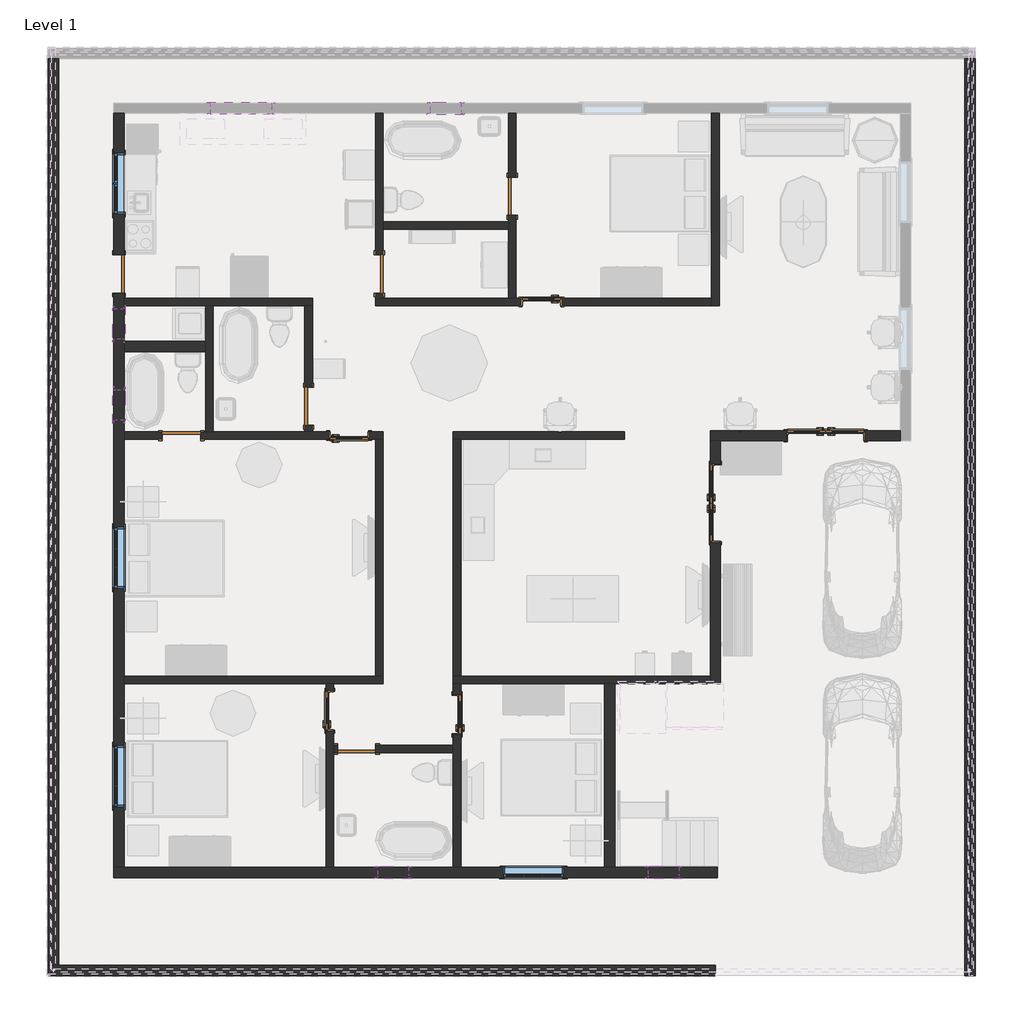
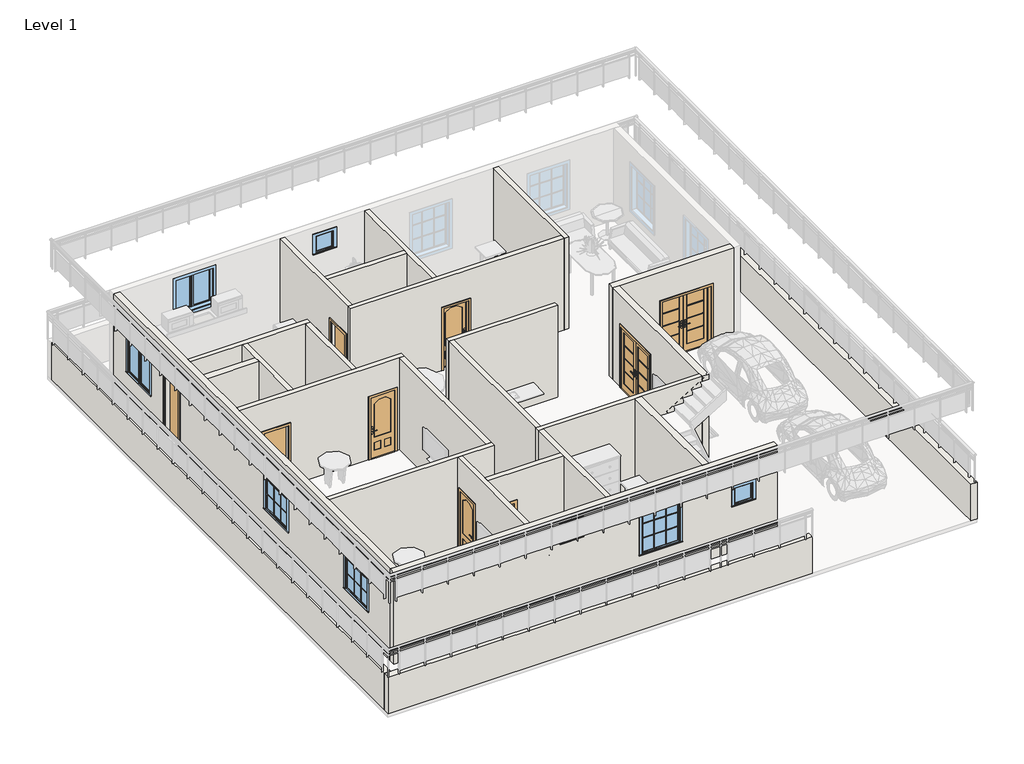
# One storey, part 1 of 6: 26 walls, 12 doors, 10 windows.
"""IFC4 building model written with IfcOpenShell, lengths in millimetres."""

from ifc_helpers import new_model, si_unit, frame, origin, origin_with_axes, place, context, project, spatial, polyline, outline, extrude, faceted_brep, transform, mapped, element, save
from components import door_14b9be53, door_4b146b56, door_b03bd389, door_c31ea698, door_1a782ffc, door_059fdd7e, door_255cab33, window_cfa1ffdd, window_0862ab64, window_3f0c7be2, window_e41d21a6

model = new_model("IFC4")

# Units and contexts
model_context = context("Model", 3, world=origin())
ifc_project = project(units=[si_unit("LENGTHUNIT", "METRE", prefix="MILLI")], contexts=[model_context])

# Site, building, storey
site = spatial("IfcSite", under=ifc_project)
building = spatial("IfcBuilding", under=site)
storey = spatial("IfcBuildingStorey", under=building, Name="Level 1", Elevation=0.0)

# Doors
placement = place(None, origin())
door_shape = door_14b9be53(model_context)
element("IfcDoor", 1, ObjectType="30\" x 80\"", at=placement, inside=storey, context=model_context, shape_type="MappedRepresentation", body=[
    mapped(door_shape, transform((266.8347674, 715.5758265, 0.0), x_axis=(0.0, -1.0, 0.0), y_axis=(1.0, 0.0, 0.0), z_axis=(0.0, 0.0, 1.0))),
])
element("IfcDoor", 2, ObjectType="30\" x 80\"", at=placement, inside=storey, context=model_context, shape_type="MappedRepresentation", body=[
    mapped(door_shape, transform((-1889.9594754, 6275.0008265, 0.0), x_axis=(-1.0, 0.0, 0.0), y_axis=(0.0, -1.0, 0.0), z_axis=(0.0, 0.0, 1.0))),
])
element("IfcDoor", 3, ObjectType="30\" x 80\"", at=placement, inside=storey, context=model_context, shape_type="MappedRepresentation", body=[
    mapped(door_shape, transform((1950.8212819, 8948.3508265, 0.0), x_axis=(1.0, 0.0, 0.0), y_axis=(0.0, 1.0, 0.0), z_axis=(0.0, 0.0, 1.0))),
])
door_2_shape = door_4b146b56(model_context)
element("IfcDoor", 4, ObjectType="30\" x 80\"", at=placement, inside=storey, context=model_context, shape_type="MappedRepresentation", body=[
    mapped(door_2_shape, transform((-2279.5152326, 791.7758265, 0.0), x_axis=(0.0, -1.0, 0.0), y_axis=(1.0, 0.0, 0.0), z_axis=(0.0, 0.0, 1.0))),
])
door_3_shape = door_b03bd389(model_context)
element("IfcDoor", 5, ObjectType="Door-Exterior-Double-Full Glass-Wood_Clad : 60\" x 80\"", at=placement, inside=storey, context=model_context, shape_type="MappedRepresentation", body=[
    mapped(door_3_shape, transform((7622.3405246, 6281.3508265, 0.0), x_axis=(1.0, 0.0, 0.0), y_axis=(0.0, 1.0, 0.0), z_axis=(0.0, 0.0, 1.0))),
])
element("IfcDoor", 6, ObjectType="Door-Exterior-Double-Full Glass-Wood_Clad : 60\" x 80\"", at=placement, inside=storey, context=model_context, shape_type="MappedRepresentation", body=[
    mapped(door_3_shape, transform((5416.6847674, 4931.9758265, 0.0), x_axis=(0.0, 1.0, 0.0), y_axis=(-1.0, 0.0, 0.0), z_axis=(0.0, 0.0, 1.0))),
])
door_4_shape = door_c31ea698(model_context)
element("IfcDoor", 7, ObjectType="Door-Single-Panel : 30\" x 80\"", at=placement, inside=storey, context=model_context, shape_type="MappedRepresentation", body=[
    mapped(door_4_shape, transform((-1285.7402326, 9503.9758265, 0.0), x_axis=(0.0, -1.0, 0.0), y_axis=(1.0, 0.0, 0.0), z_axis=(0.0, 0.0, 1.0))),
])
door_5_shape = door_1a782ffc(model_context)
element("IfcDoor", 8, ObjectType="Door-Single-Panel : 30\" x 80\"", at=placement, inside=storey, context=model_context, shape_type="MappedRepresentation", body=[
    mapped(door_5_shape, transform((-6481.9787181, 9503.9758265, 0.0), x_axis=(0.0, -1.0, 0.0), y_axis=(1.0, 0.0, 0.0), z_axis=(0.0, 0.0, 1.0))),
])
door_6_shape = door_059fdd7e(model_context)
element("IfcDoor", 9, ObjectType="Single-Flush : 30\" x 80\"", at=placement, inside=storey, context=model_context, shape_type="MappedRepresentation", body=[
    mapped(door_6_shape, transform((-5237.3787181, 6278.1758265, 0.0), x_axis=(1.0, 0.0, 0.0), y_axis=(0.0, 1.0, 0.0), z_axis=(0.0, 0.0, 1.0))),
])
element("IfcDoor", 10, ObjectType="Single-Flush : 30\" x 80\"", at=placement, inside=storey, context=model_context, shape_type="MappedRepresentation", body=[
    mapped(door_6_shape, transform((-1742.9402326, 29.7758265, 0.0), x_axis=(-1.0, 0.0, 0.0), y_axis=(0.0, -1.0, 0.0), z_axis=(0.0, 0.0, 1.0))),
])
door_7_shape = door_255cab33(model_context)
element("IfcDoor", 11, ObjectType="Single-Flush : 30\" x 80\"", at=placement, inside=storey, context=model_context, shape_type="MappedRepresentation", body=[
    mapped(door_7_shape, transform((-2697.3787181, 6862.3758265, 0.0), x_axis=(0.0, -1.0, 0.0), y_axis=(1.0, 0.0, 0.0), z_axis=(0.0, 0.0, 1.0))),
])
element("IfcDoor", 12, ObjectType="Single-Flush : 30\" x 80\"", at=placement, inside=storey, context=model_context, shape_type="MappedRepresentation", body=[
    mapped(door_7_shape, transform((1366.6212819, 11053.3758265, 0.0), x_axis=(0.0, -1.0, 0.0), y_axis=(1.0, 0.0, 0.0), z_axis=(0.0, 0.0, 1.0))),
])

# Walls
element("IfcWall", 13, at=placement, inside=storey, context=model_context, shape_type="SweptSolid", body=[
    extrude(outline(polyline([(10398.2597674, -4490.3366944), (10398.2597674, 13797.6633056), (10601.4597674, 13797.6633056), (10601.4597674, -4490.3366944), (10398.2597674, -4490.3366944)])), origin_with_axes(), (0.0, 0.0, 1.0), 1219.2),
])
element("IfcWall", 14, at=placement, inside=storey, context=model_context, shape_type="SweptSolid", body=[
    extrude(outline(polyline([(-7686.5402326, 13797.6633056), (-7686.5402326, -4287.1366944), (-7889.7402326, -4287.1366944), (-7889.7402326, 13797.6633056), (-7686.5402326, 13797.6633056)])), origin_with_axes(), (0.0, 0.0, 1.0), 1219.2),
])
element("IfcWall", 15, at=placement, inside=storey, context=model_context, shape_type="Brep", body=[
    faceted_brep([(5419.8597674, -4287.1366944, 0.0), (-7686.5402326, -4287.1366944, 0.0), (-7889.7402326, -4287.1366944, 0.0), (-7889.7402326, -4287.1366944, 1219.2), (-7686.5402326, -4287.1366944, 1219.2), (5419.8597674, -4287.1366944, 1219.2), (5419.8597674, -4490.3366944, 0.0), (5419.8597674, -4490.3366944, 1219.2), (-7889.7402326, -4490.3366944, 1219.2), (-7889.7402326, -4490.3366944, 0.0)], [[[0, 1, 2, 3, 4, 5]], [[6, 7, 8, 9]], [[3, 2, 9, 8]], [[2, 1, 0, 6, 9]], [[5, 4, 3, 8, 7]], [[0, 5, 7, 6]]]),
])
element("IfcWall", 16, ObjectType="Generic - 8\"", at=placement, inside=storey, context=model_context, shape_type="Brep", body=[
    faceted_brep([(-6380.3787181, -2332.4241735, 0.0), (-6380.3787181, 1325.1758265, 0.0), (-6380.3787181, 1477.5758265, 0.0), (-6380.3787181, 6201.9758265, 0.0), (-6380.3787181, 6354.3758265, 0.0), (-6380.3787181, 7954.5758265, 0.0), (-6380.3787181, 8157.7758265, 0.0), (-6380.3787181, 8868.9758265, 0.0), (-6380.3787181, 9021.3758265, 0.0), (-6380.3787181, 9122.9758265, 0.0), (-6380.3787181, 9122.9758265, 2032.0), (-6380.3787181, 9884.9758265, 2032.0), (-6380.3787181, 9884.9758265, 0.0), (-6380.3787181, 12704.3758265, 0.0), (-6380.3787181, 12704.3758265, 3048.0), (-6380.3787181, 9021.3758265, 3048.0), (-6380.3787181, 8868.9758265, 3048.0), (-6380.3787181, 8157.7758265, 3048.0), (-6380.3787181, 7954.5758265, 3048.0), (-6380.3787181, 6354.3758265, 3048.0), (-6380.3787181, 6201.9758265, 3048.0), (-6380.3787181, 1477.5758265, 3048.0), (-6380.3787181, 1325.1758265, 3048.0), (-6380.3787181, -2332.4241735, 3048.0), (-6380.3787181, 93.2758265, 2438.4), (-6380.3787181, 93.2758265, 914.4), (-6380.3787181, -1125.9241735, 914.4), (-6380.3787181, -1125.9241735, 2438.4), (-6380.3787181, 4449.3758265, 2438.4), (-6380.3787181, 4449.3758265, 914.4), (-6380.3787181, 3230.1758265, 914.4), (-6380.3787181, 3230.1758265, 2438.4), (-6380.3787181, 11916.9758265, 2133.6), (-6380.3787181, 11916.9758265, 914.4), (-6380.3787181, 10697.7758265, 914.4), (-6380.3787181, 10697.7758265, 2133.6), (-6380.3787181, 7192.5758265, 2768.6), (-6380.3787181, 7192.5758265, 2159.0), (-6380.3787181, 6582.9758265, 2159.0), (-6380.3787181, 6582.9758265, 2768.6), (-6380.3787181, 8195.8758265, 2768.6), (-6380.3787181, 8805.4758265, 2768.6), (-6380.3787181, 8805.4758265, 2159.0), (-6380.3787181, 8195.8758265, 2159.0), (-6583.5787181, 9122.9758265, 2032.0), (-6583.5787181, 9122.9758265, 0.0), (-6583.5787181, -2332.4241735, 0.0), (-6583.5787181, -2332.4241735, 3048.0), (-6583.5787181, 12704.3758265, 3048.0), (-6583.5787181, 12704.3758265, 0.0), (-6583.5787181, 9884.9758265, 0.0), (-6583.5787181, 9884.9758265, 2032.0), (-6583.5787181, 93.2758265, 2438.4), (-6583.5787181, -1125.9241735, 2438.4), (-6583.5787181, -1125.9241735, 914.4), (-6583.5787181, 93.2758265, 914.4), (-6583.5787181, 4449.3758265, 2438.4), (-6583.5787181, 3230.1758265, 2438.4), (-6583.5787181, 3230.1758265, 914.4), (-6583.5787181, 4449.3758265, 914.4), (-6583.5787181, 11916.9758265, 2133.6), (-6583.5787181, 10697.7758265, 2133.6), (-6583.5787181, 10697.7758265, 914.4), (-6583.5787181, 11916.9758265, 914.4), (-6583.5787181, 7192.5758265, 2768.6), (-6583.5787181, 6582.9758265, 2768.6), (-6583.5787181, 6582.9758265, 2159.0), (-6583.5787181, 7192.5758265, 2159.0), (-6583.5787181, 8195.8758265, 2768.6), (-6583.5787181, 8195.8758265, 2159.0), (-6583.5787181, 8805.4758265, 2159.0), (-6583.5787181, 8805.4758265, 2768.6)], [[[0, 1, 2, 3, 4, 5, 6, 7, 8, 9, 10, 11, 12, 13, 14, 15, 16, 17, 18, 19, 20, 21, 22, 23], [24, 25, 26, 27], [28, 29, 30, 31], [32, 33, 34, 35], [36, 37, 38, 39], [40, 41, 42, 43]], [[44, 45, 46, 47, 48, 49, 50, 51], [52, 53, 54, 55], [56, 57, 58, 59], [60, 61, 62, 63], [64, 65, 66, 67], [68, 69, 70, 71]], [[50, 49, 13, 12]], [[46, 45, 9, 8, 7, 6, 5, 4, 3, 2, 1, 0]], [[14, 13, 49, 48]], [[0, 23, 47, 46]], [[10, 9, 45, 44]], [[11, 10, 44, 51]], [[12, 11, 51, 50]], [[25, 24, 52, 55]], [[26, 25, 55, 54]], [[27, 26, 54, 53]], [[24, 27, 53, 52]], [[29, 28, 56, 59]], [[30, 29, 59, 58]], [[31, 30, 58, 57]], [[28, 31, 57, 56]], [[33, 32, 60, 63]], [[34, 33, 63, 62]], [[35, 34, 62, 61]], [[32, 35, 61, 60]], [[37, 36, 64, 67]], [[38, 37, 67, 66]], [[39, 38, 66, 65]], [[36, 39, 65, 64]], [[69, 68, 40, 43]], [[70, 69, 43, 42]], [[71, 70, 42, 41]], [[68, 71, 41, 40]], [[23, 22, 21, 20, 19, 18, 17, 16, 15, 14, 48, 47]]]),
])
element("IfcWall", 17, ObjectType="Generic - 8\"", at=placement, inside=storey, context=model_context, shape_type="Brep", body=[
    faceted_brep([(9113.6212819, 6379.7758265, 3048.0), (9113.6212819, 6379.7758265, 0.0), (8409.7405246, 6379.7758265, 0.0), (8409.7405246, 6379.7758265, 2057.4), (6834.9405246, 6379.7758265, 2057.4), (6834.9405246, 6379.7758265, 0.0), (5318.2597674, 6379.7758265, 0.0), (5318.2597674, 6379.7758265, 3048.0), (9113.6212819, 6176.5758265, 0.0), (9113.6212819, 6176.5758265, 3048.0), (5521.4597674, 6176.5758265, 3048.0), (5318.2597674, 6176.5758265, 3048.0), (5318.2597674, 6176.5758265, 0.0), (5521.4597674, 6176.5758265, 0.0), (6834.9405246, 6176.5758265, 0.0), (6834.9405246, 6176.5758265, 2057.4), (8409.7405246, 6176.5758265, 2057.4), (8409.7405246, 6176.5758265, 0.0)], [[[0, 1, 2, 3, 4, 5, 6, 7]], [[8, 9, 10, 11, 12, 13, 14, 15, 16, 17]], [[1, 8, 17, 2]], [[12, 6, 5, 14, 13]], [[1, 0, 9, 8]], [[7, 6, 12, 11]], [[16, 3, 2, 17]], [[3, 16, 15, 4]], [[4, 15, 14, 5]], [[0, 7, 11, 10, 9]]]),
])
element("IfcWall", 18, ObjectType="Generic - 8\"", at=placement, inside=storey, context=model_context, shape_type="Brep", body=[
    faceted_brep([(5456.0212819, -2332.4241735, 0.0), (3413.2597674, -2332.4241735, 0.0), (3210.0597674, -2332.4241735, 0.0), (339.8597674, -2332.4241735, 0.0), (187.4597674, -2332.4241735, 0.0), (-2200.1402326, -2332.4241735, 0.0), (-2352.5402326, -2332.4241735, 0.0), (-6380.3787181, -2332.4241735, 0.0), (-6583.5787181, -2332.4241735, 0.0), (-6583.5787181, -2332.4241735, 3048.0), (-6380.3787181, -2332.4241735, 3048.0), (-2352.5402326, -2332.4241735, 3048.0), (-2200.1402326, -2332.4241735, 3048.0), (187.4597674, -2332.4241735, 3048.0), (339.8597674, -2332.4241735, 3048.0), (3210.0597674, -2332.4241735, 3048.0), (3413.2597674, -2332.4241735, 3048.0), (5456.0212819, -2332.4241735, 3048.0), (1178.0597674, -2332.4241735, 2438.4), (1178.0597674, -2332.4241735, 914.4), (2397.2597674, -2332.4241735, 914.4), (2397.2597674, -2332.4241735, 2438.4), (-1311.1402326, -2332.4241735, 2768.6), (-1311.1402326, -2332.4241735, 2159.0), (-701.5402326, -2332.4241735, 2159.0), (-701.5402326, -2332.4241735, 2768.6), (4079.0405246, -2332.4241735, 2133.6), (4079.0405246, -2332.4241735, 1524.0), (4688.6405246, -2332.4241735, 1524.0), (4688.6405246, -2332.4241735, 2133.6), (5456.0212819, -2535.6241735, 0.0), (5456.0212819, -2535.6241735, 3048.0), (-6583.5787181, -2535.6241735, 3048.0), (-6583.5787181, -2535.6241735, 0.0), (1178.0597674, -2535.6241735, 2438.4), (2397.2597674, -2535.6241735, 2438.4), (2397.2597674, -2535.6241735, 914.4), (1178.0597674, -2535.6241735, 914.4), (-1311.1402326, -2535.6241735, 2768.6), (-701.5402326, -2535.6241735, 2768.6), (-701.5402326, -2535.6241735, 2159.0), (-1311.1402326, -2535.6241735, 2159.0), (4079.0405246, -2535.6241735, 2133.6), (4688.6405246, -2535.6241735, 2133.6), (4688.6405246, -2535.6241735, 1524.0), (4079.0405246, -2535.6241735, 1524.0)], [[[0, 1, 2, 3, 4, 5, 6, 7, 8, 9, 10, 11, 12, 13, 14, 15, 16, 17], [18, 19, 20, 21], [22, 23, 24, 25], [26, 27, 28, 29]], [[30, 31, 32, 33], [34, 35, 36, 37], [38, 39, 40, 41], [42, 43, 44, 45]], [[8, 7, 6, 5, 4, 3, 2, 1, 0, 30, 33]], [[0, 17, 31, 30]], [[9, 8, 33, 32]], [[19, 18, 34, 37]], [[20, 19, 37, 36]], [[21, 20, 36, 35]], [[18, 21, 35, 34]], [[23, 22, 38, 41]], [[24, 23, 41, 40]], [[25, 24, 40, 39]], [[22, 25, 39, 38]], [[27, 26, 42, 45]], [[28, 27, 45, 44]], [[29, 28, 44, 43]], [[26, 29, 43, 42]], [[17, 16, 15, 14, 13, 12, 11, 10, 9, 32, 31]]]),
])
element("IfcWall", 19, ObjectType="Generic - 8\"", at=placement, inside=storey, context=model_context, shape_type="SweptSolid", body=[
    extrude(outline(polyline([(3210.0597674, -2332.4241735), (3210.0597674, 1325.1758265), (3413.2597674, 1325.1758265), (3413.2597674, -2332.4241735), (3210.0597674, -2332.4241735)])), origin_with_axes(), (0.0, 0.0, 1.0), 3048.0),
])
element("IfcWall", 20, ObjectType="Generic - 8\"", at=placement, inside=storey, context=model_context, shape_type="Brep", body=[
    faceted_brep([(5521.4597674, 1325.1758265, 3048.0), (5521.4597674, 1325.1758265, 0.0), (5521.4597674, 4144.5758265, 0.0), (5521.4597674, 4144.5758265, 2057.4), (5521.4597674, 5719.3758265, 2057.4), (5521.4597674, 5719.3758265, 0.0), (5521.4597674, 6176.5758265, 0.0), (5521.4597674, 6176.5758265, 3048.0), (5318.2597674, 1325.1758265, 0.0), (5318.2597674, 1325.1758265, 3048.0), (5318.2597674, 1477.5758265, 3048.0), (5318.2597674, 6176.5758265, 3048.0), (5318.2597674, 6176.5758265, 0.0), (5318.2597674, 5719.3758265, 0.0), (5318.2597674, 5719.3758265, 2057.4), (5318.2597674, 4144.5758265, 2057.4), (5318.2597674, 4144.5758265, 0.0), (5318.2597674, 1477.5758265, 0.0)], [[[0, 1, 2, 3, 4, 5, 6, 7]], [[8, 9, 10, 11, 12, 13, 14, 15, 16, 17]], [[1, 8, 17, 16, 2]], [[12, 6, 5, 13]], [[1, 0, 9, 8]], [[7, 6, 12, 11]], [[4, 14, 13, 5]], [[14, 4, 3, 15]], [[15, 3, 2, 16]], [[0, 7, 11, 10, 9]]]),
])
element("IfcWall", 21, ObjectType="Generic - 8\"", at=placement, inside=storey, context=model_context, shape_type="SweptSolid", body=[
    extrude(outline(polyline([(-6380.3787181, 8157.7758265), (-4754.7787181, 8157.7758265), (-4754.7787181, 7954.5758265), (-6380.3787181, 7954.5758265), (-6380.3787181, 8157.7758265)])), origin_with_axes(), (0.0, 0.0, 1.0), 3048.0),
])
element("IfcWall", 22, ObjectType="INNER WALL", at=placement, inside=storey, context=model_context, shape_type="Brep", body=[
    faceted_brep([(5318.2597674, 1477.5758265, 0.0), (339.8597674, 1477.5758265, 0.0), (187.4597674, 1477.5758265, 0.0), (187.4597674, 1477.5758265, 3048.0), (339.8597674, 1477.5758265, 3048.0), (5318.2597674, 1477.5758265, 3048.0), (5318.2597674, 1325.1758265, 0.0), (5318.2597674, 1325.1758265, 3048.0), (3413.2597674, 1325.1758265, 3048.0), (3210.0597674, 1325.1758265, 3048.0), (339.8597674, 1325.1758265, 3048.0), (187.4597674, 1325.1758265, 3048.0), (187.4597674, 1325.1758265, 0.0), (339.8597674, 1325.1758265, 0.0), (3210.0597674, 1325.1758265, 0.0), (3413.2597674, 1325.1758265, 0.0)], [[[0, 1, 2, 3, 4, 5]], [[6, 7, 8, 9, 10, 11, 12, 13, 14, 15]], [[2, 1, 0, 6, 15, 14, 13, 12]], [[3, 2, 12, 11]], [[0, 5, 7, 6]], [[5, 4, 3, 11, 10, 9, 8, 7]]]),
])
element("IfcWall", 23, ObjectType="INNER WALL", at=placement, inside=storey, context=model_context, shape_type="Brep", body=[
    faceted_brep([(187.4597674, -2332.4241735, 0.0), (187.4597674, -2332.4241735, 3048.0), (187.4597674, -46.4241735, 3048.0), (187.4597674, 105.9758265, 3048.0), (187.4597674, 1325.1758265, 3048.0), (187.4597674, 1325.1758265, 0.0), (187.4597674, 1121.9758265, 0.0), (187.4597674, 1121.9758265, 2057.4), (187.4597674, 309.1758265, 2057.4), (187.4597674, 309.1758265, 0.0), (187.4597674, 105.9758265, 0.0), (187.4597674, -46.4241735, 0.0), (339.8597674, -2332.4241735, 3048.0), (339.8597674, -2332.4241735, 0.0), (339.8597674, 309.1758265, 0.0), (339.8597674, 309.1758265, 2057.4), (339.8597674, 1121.9758265, 2057.4), (339.8597674, 1121.9758265, 0.0), (339.8597674, 1325.1758265, 0.0), (339.8597674, 1325.1758265, 3048.0)], [[[0, 1, 2, 3, 4, 5, 6, 7, 8, 9, 10, 11]], [[12, 13, 14, 15, 16, 17, 18, 19]], [[13, 0, 11, 10, 9, 14]], [[5, 18, 17, 6]], [[1, 0, 13, 12]], [[5, 4, 19, 18]], [[8, 15, 14, 9]], [[15, 8, 7, 16]], [[16, 7, 6, 17]], [[4, 3, 2, 1, 12, 19]]]),
])
element("IfcWall", 24, ObjectType="INNER WALL", at=placement, inside=storey, context=model_context, shape_type="Brep", body=[
    faceted_brep([(-2352.5402326, -2332.4241735, 0.0), (-2352.5402326, -2332.4241735, 3048.0), (-2352.5402326, 1325.1758265, 3048.0), (-2352.5402326, 1325.1758265, 0.0), (-2352.5402326, 1198.1758265, 0.0), (-2352.5402326, 1198.1758265, 2057.4), (-2352.5402326, 385.3758265, 2057.4), (-2352.5402326, 385.3758265, 0.0), (-2200.1402326, -2332.4241735, 3048.0), (-2200.1402326, -2332.4241735, 0.0), (-2200.1402326, -46.4241735, 0.0), (-2200.1402326, 105.9758265, 0.0), (-2200.1402326, 385.3758265, 0.0), (-2200.1402326, 385.3758265, 2057.4), (-2200.1402326, 1198.1758265, 2057.4), (-2200.1402326, 1198.1758265, 0.0), (-2200.1402326, 1325.1758265, 0.0), (-2200.1402326, 1325.1758265, 3048.0), (-2200.1402326, 105.9758265, 3048.0), (-2200.1402326, -46.4241735, 3048.0)], [[[0, 1, 2, 3, 4, 5, 6, 7]], [[8, 9, 10, 11, 12, 13, 14, 15, 16, 17, 18, 19]], [[3, 16, 15, 4]], [[9, 0, 7, 12, 11, 10]], [[1, 0, 9, 8]], [[3, 2, 17, 16]], [[6, 13, 12, 7]], [[13, 6, 5, 14]], [[14, 5, 4, 15]], [[2, 1, 8, 19, 18, 17]]]),
])
element("IfcWall", 25, ObjectType="INNER WALL", at=placement, inside=storey, context=model_context, shape_type="SweptSolid", body=[
    extrude(outline(polyline([(339.8597674, 6201.9758265), (339.8597674, 1477.5758265), (187.4597674, 1477.5758265), (187.4597674, 6201.9758265), (339.8597674, 6201.9758265)])), origin_with_axes(), (0.0, 0.0, 1.0), 3048.0),
])
element("IfcWall", 26, ObjectType="INNER WALL", at=placement, inside=storey, context=model_context, shape_type="SweptSolid", body=[
    extrude(outline(polyline([(-1361.9402326, 1477.5758265), (-1361.9402326, 6201.9758265), (-1209.5402326, 6201.9758265), (-1209.5402326, 1477.5758265), (-1361.9402326, 1477.5758265)])), origin_with_axes(), (0.0, 0.0, 1.0), 3048.0),
])
element("IfcWall", 27, ObjectType="INNER WALL", at=placement, inside=storey, context=model_context, shape_type="Brep", body=[
    faceted_brep([(-1209.5402326, 1477.5758265, 0.0), (-1361.9402326, 1477.5758265, 0.0), (-6380.3787181, 1477.5758265, 0.0), (-6380.3787181, 1477.5758265, 3048.0), (-1361.9402326, 1477.5758265, 3048.0), (-1209.5402326, 1477.5758265, 3048.0), (-1209.5402326, 1325.1758265, 0.0), (-1209.5402326, 1325.1758265, 3048.0), (-2200.1402326, 1325.1758265, 3048.0), (-2352.5402326, 1325.1758265, 3048.0), (-6380.3787181, 1325.1758265, 3048.0), (-6380.3787181, 1325.1758265, 0.0), (-2352.5402326, 1325.1758265, 0.0), (-2200.1402326, 1325.1758265, 0.0)], [[[0, 1, 2, 3, 4, 5]], [[6, 7, 8, 9, 10, 11, 12, 13]], [[2, 1, 0, 6, 13, 12, 11]], [[3, 2, 11, 10]], [[0, 5, 7, 6]], [[5, 4, 3, 10, 9, 8, 7]]]),
])
element("IfcWall", 28, ObjectType="INNER WALL", at=placement, inside=storey, context=model_context, shape_type="Brep", body=[
    faceted_brep([(-6380.3787181, 6354.3758265, 0.0), (-6380.3787181, 6354.3758265, 3048.0), (-4754.7787181, 6354.3758265, 3048.0), (-4602.3787181, 6354.3758265, 3048.0), (-2773.5787181, 6354.3758265, 3048.0), (-2621.1787181, 6354.3758265, 3048.0), (-1209.5402326, 6354.3758265, 3048.0), (-1209.5402326, 6354.3758265, 0.0), (-1483.5594754, 6354.3758265, 0.0), (-1483.5594754, 6354.3758265, 2057.4), (-2296.3594754, 6354.3758265, 2057.4), (-2296.3594754, 6354.3758265, 0.0), (-2621.1787181, 6354.3758265, 0.0), (-2773.5787181, 6354.3758265, 0.0), (-4602.3787181, 6354.3758265, 0.0), (-4754.7787181, 6354.3758265, 0.0), (-4856.3787181, 6354.3758265, 0.0), (-4856.3787181, 6354.3758265, 2032.0), (-5618.3787181, 6354.3758265, 2032.0), (-5618.3787181, 6354.3758265, 0.0), (-6380.3787181, 6201.9758265, 3048.0), (-6380.3787181, 6201.9758265, 0.0), (-5618.3787181, 6201.9758265, 0.0), (-5618.3787181, 6201.9758265, 2032.0), (-4856.3787181, 6201.9758265, 2032.0), (-4856.3787181, 6201.9758265, 0.0), (-2296.3594754, 6201.9758265, 0.0), (-2296.3594754, 6201.9758265, 2057.4), (-1483.5594754, 6201.9758265, 2057.4), (-1483.5594754, 6201.9758265, 0.0), (-1361.9402326, 6201.9758265, 0.0), (-1209.5402326, 6201.9758265, 0.0), (-1209.5402326, 6201.9758265, 3048.0), (-1361.9402326, 6201.9758265, 3048.0)], [[[0, 1, 2, 3, 4, 5, 6, 7, 8, 9, 10, 11, 12, 13, 14, 15, 16, 17, 18, 19]], [[20, 21, 22, 23, 24, 25, 26, 27, 28, 29, 30, 31, 32, 33]], [[21, 0, 19, 22]], [[7, 31, 30, 29, 8]], [[25, 16, 15, 14, 13, 12, 11, 26]], [[1, 0, 21, 20]], [[7, 6, 32, 31]], [[17, 16, 25, 24]], [[18, 17, 24, 23]], [[19, 18, 23, 22]], [[10, 27, 26, 11]], [[27, 10, 9, 28]], [[28, 9, 8, 29]], [[6, 5, 4, 3, 2, 1, 20, 33, 32]]]),
])
element("IfcWall", 29, ObjectType="INNER WALL", at=placement, inside=storey, context=model_context, shape_type="SweptSolid", body=[
    extrude(outline(polyline([(0.0, -2200.1402326), (0.0, -2123.9402326), (2032.0, -2123.9402326), (2032.0, -1361.9402326), (0.0, -1361.9402326), (0.0, 187.4597674), (3048.0, 187.4597674), (3048.0, -2200.1402326), (0.0, -2200.1402326)])), frame((0.0, -46.4241735, 0.0), z_axis=(0.0, 1.0, 0.0), x_axis=(0.0, 0.0, 1.0)), (0.0, 0.0, 1.0), 152.4),
])
element("IfcWall", 30, ObjectType="INNER WALL", at=placement, inside=storey, context=model_context, shape_type="Brep", body=[
    faceted_brep([(-6380.3787181, 8868.9758265, 0.0), (-4754.7787181, 8868.9758265, 0.0), (-4602.3787181, 8868.9758265, 0.0), (-2773.5787181, 8868.9758265, 0.0), (-2621.1787181, 8868.9758265, 0.0), (-2621.1787181, 8868.9758265, 3048.0), (-2773.5787181, 8868.9758265, 3048.0), (-4602.3787181, 8868.9758265, 3048.0), (-4754.7787181, 8868.9758265, 3048.0), (-6380.3787181, 8868.9758265, 3048.0), (-6380.3787181, 9021.3758265, 0.0), (-6380.3787181, 9021.3758265, 3048.0), (-2621.1787181, 9021.3758265, 3048.0), (-2621.1787181, 9021.3758265, 0.0)], [[[0, 1, 2, 3, 4, 5, 6, 7, 8, 9]], [[10, 11, 12, 13]], [[4, 3, 2, 1, 0, 10, 13]], [[0, 9, 11, 10]], [[5, 4, 13, 12]], [[9, 8, 7, 6, 5, 12, 11]]]),
])
element("IfcWall", 31, ObjectType="INNER WALL", at=placement, inside=storey, context=model_context, shape_type="Brep", body=[
    faceted_brep([(-4754.7787181, 8868.9758265, 0.0), (-4754.7787181, 8157.7758265, 0.0), (-4754.7787181, 7954.5758265, 0.0), (-4754.7787181, 6354.3758265, 0.0), (-4754.7787181, 6354.3758265, 3048.0), (-4754.7787181, 7954.5758265, 3048.0), (-4754.7787181, 8157.7758265, 3048.0), (-4754.7787181, 8868.9758265, 3048.0), (-4602.3787181, 8868.9758265, 0.0), (-4602.3787181, 8868.9758265, 3048.0), (-4602.3787181, 6354.3758265, 3048.0), (-4602.3787181, 6354.3758265, 0.0)], [[[0, 1, 2, 3, 4, 5, 6, 7]], [[8, 9, 10, 11]], [[3, 2, 1, 0, 8, 11]], [[4, 3, 11, 10]], [[0, 7, 9, 8]], [[7, 6, 5, 4, 10, 9]]]),
])
element("IfcWall", 32, ObjectType="INNER WALL", at=placement, inside=storey, context=model_context, shape_type="SweptSolid", body=[
    extrude(outline(polyline([(6481.3758265, 2032.0), (6481.3758265, 0.0), (6354.3758265, 0.0), (6354.3758265, 3048.0), (8868.9758265, 3048.0), (8868.9758265, 0.0), (7243.3758265, 0.0), (7243.3758265, 2032.0), (6481.3758265, 2032.0)])), frame((-2773.5787181, 0.0, 0.0), z_axis=(1.0, 0.0, 0.0), x_axis=(0.0, 1.0, 0.0)), (0.0, 0.0, 1.0), 152.4),
])
element("IfcWall", 33, ObjectType="INNER WALL", at=placement, inside=storey, context=model_context, shape_type="Brep", body=[
    faceted_brep([(-1209.5402326, 9021.3758265, 0.0), (-1209.5402326, 9122.9758265, 0.0), (-1209.5402326, 9122.9758265, 2032.0), (-1209.5402326, 9884.9758265, 2032.0), (-1209.5402326, 9884.9758265, 0.0), (-1209.5402326, 10392.9758265, 0.0), (-1209.5402326, 10545.3758265, 0.0), (-1209.5402326, 12704.3758265, 0.0), (-1209.5402326, 12704.3758265, 3048.0), (-1209.5402326, 10545.3758265, 3048.0), (-1209.5402326, 10392.9758265, 3048.0), (-1209.5402326, 9021.3758265, 3048.0), (-1361.9402326, 9122.9758265, 2032.0), (-1361.9402326, 9122.9758265, 0.0), (-1361.9402326, 9021.3758265, 0.0), (-1361.9402326, 9021.3758265, 3048.0), (-1361.9402326, 12704.3758265, 3048.0), (-1361.9402326, 12704.3758265, 0.0), (-1361.9402326, 9884.9758265, 0.0), (-1361.9402326, 9884.9758265, 2032.0)], [[[0, 1, 2, 3, 4, 5, 6, 7, 8, 9, 10, 11]], [[12, 13, 14, 15, 16, 17, 18, 19]], [[18, 17, 7, 6, 5, 4]], [[14, 13, 1, 0]], [[8, 7, 17, 16]], [[0, 11, 15, 14]], [[2, 1, 13, 12]], [[3, 2, 12, 19]], [[4, 3, 19, 18]], [[11, 10, 9, 8, 16, 15]]]),
])
element("IfcWall", 34, ObjectType="INNER WALL", at=placement, inside=storey, context=model_context, shape_type="Brep", body=[
    faceted_brep([(1290.4212819, 10672.3758265, 2032.0), (1290.4212819, 10672.3758265, 0.0), (1290.4212819, 10545.3758265, 0.0), (1290.4212819, 10392.9758265, 0.0), (1290.4212819, 9021.3758265, 0.0), (1290.4212819, 9021.3758265, 3048.0), (1290.4212819, 10392.9758265, 3048.0), (1290.4212819, 10545.3758265, 3048.0), (1290.4212819, 12704.3758265, 3048.0), (1290.4212819, 12704.3758265, 0.0), (1290.4212819, 11434.3758265, 0.0), (1290.4212819, 11434.3758265, 2032.0), (1442.8212819, 9021.3758265, 0.0), (1442.8212819, 10672.3758265, 0.0), (1442.8212819, 10672.3758265, 2032.0), (1442.8212819, 11434.3758265, 2032.0), (1442.8212819, 11434.3758265, 0.0), (1442.8212819, 12704.3758265, 0.0), (1442.8212819, 12704.3758265, 3048.0), (1442.8212819, 9021.3758265, 3048.0)], [[[0, 1, 2, 3, 4, 5, 6, 7, 8, 9, 10, 11]], [[12, 13, 14, 15, 16, 17, 18, 19]], [[10, 9, 17, 16]], [[4, 3, 2, 1, 13, 12]], [[9, 8, 18, 17]], [[5, 4, 12, 19]], [[14, 13, 1, 0]], [[15, 14, 0, 11]], [[16, 15, 11, 10]], [[8, 7, 6, 5, 19, 18]]]),
])
element("IfcWall", 35, ObjectType="INNER WALL", at=placement, inside=storey, context=model_context, shape_type="SweptSolid", body=[
    extrude(outline(polyline([(-1209.5402326, 10545.3758265), (1290.4212819, 10545.3758265), (1290.4212819, 10392.9758265), (-1209.5402326, 10392.9758265), (-1209.5402326, 10545.3758265)])), origin_with_axes(), (0.0, 0.0, 1.0), 3048.0),
])
element("IfcWall", 36, ObjectType="INNER WALL", at=placement, inside=storey, context=model_context, shape_type="Brep", body=[
    faceted_brep([(5496.0597674, 8868.9758265, 0.0), (5496.0597674, 12704.3758265, 0.0), (5496.0597674, 12704.3758265, 3048.0), (5496.0597674, 8868.9758265, 3048.0), (5343.6597674, 8868.9758265, 0.0), (5343.6597674, 8868.9758265, 3048.0), (5343.6597674, 9021.3758265, 3048.0), (5343.6597674, 12704.3758265, 3048.0), (5343.6597674, 12704.3758265, 0.0), (5343.6597674, 9021.3758265, 0.0)], [[[0, 1, 2, 3]], [[4, 5, 6, 7, 8, 9]], [[1, 0, 4, 9, 8]], [[2, 1, 8, 7]], [[0, 3, 5, 4]], [[3, 2, 7, 6, 5]]]),
])
element("IfcWall", 37, ObjectType="INNER WALL", at=placement, inside=storey, context=model_context, shape_type="Brep", body=[
    faceted_brep([(5343.6597674, 8868.9758265, 0.0), (5343.6597674, 8868.9758265, 3048.0), (-1361.9402326, 8868.9758265, 3048.0), (-1361.9402326, 8868.9758265, 0.0), (1544.4212819, 8868.9758265, 0.0), (1544.4212819, 8868.9758265, 2057.4), (2357.2212819, 8868.9758265, 2057.4), (2357.2212819, 8868.9758265, 0.0), (5343.6597674, 9021.3758265, 3048.0), (5343.6597674, 9021.3758265, 0.0), (2357.2212819, 9021.3758265, 0.0), (2357.2212819, 9021.3758265, 2057.4), (1544.4212819, 9021.3758265, 2057.4), (1544.4212819, 9021.3758265, 0.0), (1442.8212819, 9021.3758265, 0.0), (1290.4212819, 9021.3758265, 0.0), (-1209.5402326, 9021.3758265, 0.0), (-1361.9402326, 9021.3758265, 0.0), (-1361.9402326, 9021.3758265, 3048.0), (-1209.5402326, 9021.3758265, 3048.0), (1290.4212819, 9021.3758265, 3048.0), (1442.8212819, 9021.3758265, 3048.0)], [[[0, 1, 2, 3, 4, 5, 6, 7]], [[8, 9, 10, 11, 12, 13, 14, 15, 16, 17, 18, 19, 20, 21]], [[9, 0, 7, 10]], [[3, 17, 16, 15, 14, 13, 4]], [[1, 0, 9, 8]], [[3, 2, 18, 17]], [[6, 11, 10, 7]], [[11, 6, 5, 12]], [[12, 5, 4, 13]], [[2, 1, 8, 21, 20, 19, 18]]]),
])
element("IfcWall", 38, ObjectType="INNER WALL", at=placement, inside=storey, context=model_context, shape_type="Brep", body=[
    faceted_brep([(3601.8212819, 6354.3758265, 0.0), (187.4597674, 6354.3758265, 0.0), (187.4597674, 6354.3758265, 3048.0), (3601.8212819, 6354.3758265, 3048.0), (3601.8212819, 6201.9758265, 0.0), (3601.8212819, 6201.9758265, 3048.0), (339.8597674, 6201.9758265, 3048.0), (187.4597674, 6201.9758265, 3048.0), (187.4597674, 6201.9758265, 0.0), (339.8597674, 6201.9758265, 0.0)], [[[0, 1, 2, 3]], [[4, 5, 6, 7, 8, 9]], [[1, 0, 4, 9, 8]], [[0, 3, 5, 4]], [[2, 1, 8, 7]], [[3, 2, 7, 6, 5]]]),
])

# Windows
window_shape = window_cfa1ffdd(model_context)
element("IfcWindow", 39, ObjectType="Casement 3x3 with Trim : 48\" x 60\"", at=placement, inside=storey, context=model_context, shape_type="MappedRepresentation", body=[
    mapped(window_shape, transform((-6481.9787181, -516.3241735, 304.8), x_axis=(0.0, 1.0, 0.0), y_axis=(-1.0, 0.0, 0.0), z_axis=(0.0, 0.0, 1.0))),
])
element("IfcWindow", 40, ObjectType="Casement 3x3 with Trim : 48\" x 60\"", at=placement, inside=storey, context=model_context, shape_type="MappedRepresentation", body=[
    mapped(window_shape, transform((-6481.9787181, 3839.7758265, 304.8), x_axis=(0.0, 1.0, 0.0), y_axis=(-1.0, 0.0, 0.0), z_axis=(0.0, 0.0, 1.0))),
])
element("IfcWindow", 41, ObjectType="Casement 3x3 with Trim : 48\" x 60\"", at=placement, inside=storey, context=model_context, shape_type="MappedRepresentation", body=[
    mapped(window_shape, transform((1787.6597674, -2434.0241735, 304.8), x_axis=(-1.0, 0.0, 0.0), y_axis=(0.0, -1.0, 0.0), z_axis=(0.0, 0.0, 1.0))),
])
window_2_shape = window_0862ab64(model_context)
element("IfcWindow", 42, ObjectType="Casement Dbl with Trim : 48\" x 48\"", at=placement, inside=storey, context=model_context, shape_type="MappedRepresentation", body=[
    mapped(window_2_shape, transform((-4043.5787181, 12786.9258265, 711.2), x_axis=(1.0, 0.0, 0.0), y_axis=(0.0, 1.0, 0.0), z_axis=(0.0, 0.0, 1.0))),
])
element("IfcWindow", 43, ObjectType="Casement Dbl with Trim : 48\" x 48\"", at=placement, inside=storey, context=model_context, shape_type="MappedRepresentation", body=[
    mapped(window_2_shape, transform((-6462.9287181, 11307.3758265, 0.0), x_axis=(0.0, 1.0, 0.0), y_axis=(-1.0, 0.0, 0.0), z_axis=(0.0, 0.0, 1.0))),
])
window_3_shape = window_3f0c7be2(model_context)
element("IfcWindow", 44, ObjectType="Casement with Trim : 24\" x 24\"", at=placement, inside=storey, context=model_context, shape_type="MappedRepresentation", body=[
    mapped(window_3_shape, transform((4383.8405246, -2434.0241735, 609.6), x_axis=(-1.0, 0.0, 0.0), y_axis=(0.0, -1.0, 0.0), z_axis=(0.0, 0.0, 1.0))),
])
window_4_shape = window_e41d21a6(model_context)
element("IfcWindow", 45, ObjectType="Transom with Trim : 24\" x 24\"", at=placement, inside=storey, context=model_context, shape_type="MappedRepresentation", body=[
    mapped(window_4_shape, transform((-1044.4402326, -2434.0241735, 0.0), x_axis=(-1.0, 0.0, 0.0), y_axis=(0.0, -1.0, 0.0), z_axis=(0.0, 0.0, 1.0))),
])
element("IfcWindow", 46, ObjectType="Transom with Trim : 24\" x 24\"", at=placement, inside=storey, context=model_context, shape_type="MappedRepresentation", body=[
    mapped(window_4_shape, transform((-6481.9787181, 6925.8758265, 0.0), x_axis=(0.0, 1.0, 0.0), y_axis=(-1.0, 0.0, 0.0), z_axis=(0.0, 0.0, 1.0))),
])
element("IfcWindow", 47, ObjectType="Transom with Trim : 24\" x 24\"", at=placement, inside=storey, context=model_context, shape_type="MappedRepresentation", body=[
    mapped(window_4_shape, transform((-6481.9787181, 8462.5758265, 0.0), x_axis=(0.0, -1.0, 0.0), y_axis=(1.0, 0.0, 0.0), z_axis=(0.0, 0.0, 1.0))),
])
element("IfcWindow", 48, ObjectType="Transom with Trim : 24\" x 24\"", at=placement, inside=storey, context=model_context, shape_type="MappedRepresentation", body=[
    mapped(window_4_shape, transform((2.3405246, 12805.9758265, 0.0), x_axis=(-1.0, 0.0, 0.0), y_axis=(0.0, -1.0, 0.0), z_axis=(0.0, 0.0, 1.0))),
])

save(model, "model.ifc")

# Revit data of these elements
# Type "30\" x 80\""
#   Type Mark = "10"
#   Assembly Code = "B2030100"
#   Analytic Construction = "French door, wood frame with single glass"
#   Threshold Offset [instance default] = 0' - 0 1/2"
#   Thickness = 0' - 1 3/8"
#   Thermal Resistance (R) = 1.0696 (h·ft²·°F)/BTU
#   Swing Angle [instance default] = 90.00°
#   Stiles = 0' - 4 3/4"
#   Rough Width = 2' - 8"
#   Rough Height = 6' - 9"
#   Radius = 1' - 1.00625"
#   Lock Rail = 0' - 7 1/8"
#   Height = 6' - 8"
#   Width = 2' - 6"
#   Heat Transfer Coefficient (U) = 0.9350 BTU/(h·ft²·°F)
#   Door Offset [instance default] = 0' - 0"
#   Bottom Rail = 0' - 9 1/2"
#   Threshold [instance default] = yes
#   Function = 1
#   Exterior Trim [instance default] = yes
#   Trim Material = Cherry
#   Threshold Material = Cherry
#   Panel Material = Cherry
#   Glazing = Glass
#   Frame Material = Cherry
#   Door Handle Material = Aluminum
#   Visual Light Transmittance = 0
#   Solar Heat Gain Coefficient = 0
#   Wall Closure = (empty or 0)
#   Construction Type = (empty or 0)
# Type "Door-Exterior-Double-Full Glass-Wood_Clad : 60\" x 80\""
#   Type Mark = "9"
#   Assembly Code = "B2030100"
#   Analytic Construction = "French door, wood frame with double glass"
#   Top Rail = 0' - 4 11/16"
#   Threshold Offset [instance default] = 0' - 0 1/2"
#   Thickness = 0' - 1 3/8"
#   Thermal Resistance (R) = 1.9158 (h·ft²·°F)/BTU
#   Swing Angle [instance default] = 90.00°
#   Stiles = 0' - 4 3/4"
#   Rough Width = 5' - 2"
#   Rough Height = 6' - 9"
#   Panel Width = 2' - 6"
#   Door Offset [instance default] = 0' - 0"
#   Height = 6' - 8"
#   Width = 5' - 0"
#   Heat Transfer Coefficient (U) = 0.5220 BTU/(h·ft²·°F)
#   Bottom Rail = 0' - 9 1/8"
#   Exterior Trim [instance default] = yes
#   Threshold [instance default] = yes
#   Show Grill [instance default] = yes
#   Function = 1
#   Trim Material = Cherry
#   Threshold Material = Cherry
#   Panel Material = Cherry
#   Glazing = Glass
#   Frame Material = Cherry
#   Door Handle Material = Aluminum
#   Visual Light Transmittance = 0
#   Solar Heat Gain Coefficient = 0
#   Wall Closure = (empty or 0)
#   Construction Type = (empty or 0)
# Type "Door-Single-Panel : 30\" x 80\""
#   Type Mark = "8"
#   Construction Type Id = "DOOR"
#   Assembly Code = "C1020300"
#   Analytic Construction = "Wooden"
#   Thickness = 0' - 2"
#   Thermal Resistance (R) = 2.5876 (h·ft²·°F)/BTU
#   Swing Angle [instance default] = 90.00°
#   Heat Transfer Coefficient (U) = 0.3865 BTU/(h·ft²·°F)
#   Height = 6' - 8"
#   Trim Projection Ext = 0' - 1"
#   Trim Projection Int = 0' - 1"
#   Trim Width = 0' - 3"
#   Width = 2' - 6"
#   Define Thermal Properties by = 1
#   Panel Material = Wood - Birch - Solid Stained Light Low Gloss
#   Trim Material = Paint - Sienna
#   Visual Light Transmittance = 0
#   Solar Heat Gain Coefficient = 0
#   Function = (empty or 0)
#   Wall Closure = (empty or 0)
# Type "Single-Flush : 30\" x 80\""
#   Type Mark = "5"
#   Construction Type Id = "MDOOR"
#   Assembly Code = "C1020"
#   Analytic Construction = "Metal"
#   Thickness = 0' - 2"
#   Heat Transfer Coefficient (U) = 0.651978 BTU/(h·ft²·°F)
#   Height = 6' - 8"
#   Trim Projection Ext = 0' - 1"
#   Trim Projection Int = 0' - 1"
#   Trim Width = 0' - 3"
#   Width = 2' - 6"
#   Define Thermal Properties by = 1
#   Door Material = Door - Panel
#   Frame Material = Door - Frame
#   Visual Light Transmittance = 0
#   Solar Heat Gain Coefficient = 0
#   Function = (empty or 0)
#   Wall Closure = (empty or 0)
# Type
#   Assembly Code = "B2010"
#   Layers, outside or top first: 0' - 8" "Asphalt Shingle" (function 1)
# Type "Generic - 8\""
#   Assembly Code = "B2010"
#   Layers, outside or top first: 0' - 8" "Brick, Common" (function 1)
# Type "INNER WALL"
#   Assembly Code = "B2010"
#   Layers, outside or top first: 0' - 6" "Brick, Soldier Course" (function 1)
# Type "Casement 3x3 with Trim : 48\" x 60\""
#   Type Mark = "11"
#   Construction Type Id = "GSP4R"
#   Assembly Code = "B2020100"
#   Analytic Construction = "1/8 in Pilkington single glazing"
#   Visual Light Transmittance = 0.9
#   Solar Heat Gain Coefficient = 0.78
#   Heat Transfer Coefficient (U) = 0.6496 BTU/(h·ft²·°F)
#   Height = 5' - 0"
#   Default Sill Height = 2' - 0"
#   Trim Projection - Ext. = 0' - 0 1/2"
#   Trim Projection - Int. = 0' - 0 3/4"
#   Trim Width - Exterior = 0' - 3 1/2"
#   Trim Width - Interior = 0' - 3 1/2"
#   Width = 4' - 0"
#   Window Inset = 0' - 0 3/4"
#   Define Thermal Properties by = 1
#   Glass Pane Material = Glass
#   Sash Material = Sash
#   Trim Exterior Material = Trim
#   Trim Interior Material = Trim
#   Wall Closure = (empty or 0)
# Type "Casement Dbl with Trim : 48\" x 48\""
#   Type Mark = "13"
#   Construction Type Id = "GSP4R"
#   Assembly Code = "B2020100"
#   Analytic Construction = "1/8 in Pilkington single glazing"
#   Visual Light Transmittance = 0.9
#   Solar Heat Gain Coefficient = 0.78
#   Heat Transfer Coefficient (U) = 0.6496 BTU/(h·ft²·°F)
#   Height = 4' - 0"
#   Default Sill Height = 3' - 0"
#   Trim Projection - Ext. = 0' - 0 1/2"
#   Trim Projection - Int. = 0' - 0 3/4"
#   Trim Width - Exterior = 0' - 3 1/2"
#   Trim Width - Interior = 0' - 3 1/2"
#   Width = 4' - 0"
#   Window Inset = 0' - 0 3/4"
#   Define Thermal Properties by = 1
#   Glass Pane Material = Glass
#   Sash Material = Sash
#   Trim Exterior Material = Trim
#   Trim Interior Material = Trim
#   Wall Closure = (empty or 0)
# Type "Casement with Trim : 24\" x 24\""
#   Type Mark = "28"
#   Construction Type Id = "GSP4R"
#   Assembly Code = "B2020100"
#   Analytic Construction = "1/8 in Pilkington single glazing"
#   Visual Light Transmittance = 0.9
#   Solar Heat Gain Coefficient = 0.78
#   Heat Transfer Coefficient (U) = 0.6496 BTU/(h·ft²·°F)
#   Height = 2' - 0"
#   Default Sill Height = 3' - 0"
#   Trim Projection - Ext. = 0' - 0 1/2"
#   Trim Projection - Int. = 0' - 0 3/4"
#   Trim Width - Exterior = 0' - 3 1/2"
#   Trim Width - Interior = 0' - 3 1/2"
#   Width = 2' - 0"
#   Window Inset = 0' - 0 3/4"
#   Define Thermal Properties by = 1
#   Glass Pane Material = Glass
#   Sash Material = Sash
#   Trim Exterior Material = Trim
#   Trim Interior Material = Trim
#   Wall Closure = (empty or 0)
# Type "Transom with Trim : 24\" x 24\""
#   Type Mark = "16"
#   Construction Type Id = "GSP4R"
#   Assembly Code = "B2020100"
#   Analytic Construction = "1/8 in Pilkington single glazing"
#   Visual Light Transmittance = 0.9
#   Solar Heat Gain Coefficient = 0.78
#   Heat Transfer Coefficient (U) = 0.6496 BTU/(h·ft²·°F)
#   Height = 2' - 0"
#   Default Sill Height = 7' - 1"
#   Trim Projection - Ext. = 0' - 0 1/2"
#   Trim Projection - Int. = 0' - 0 3/4"
#   Trim Width - Exterior = 0' - 3 1/2"
#   Trim Width - Interior = 0' - 3 1/2"
#   Width = 2' - 0"
#   Window Inset = 0' - 0 3/4"
#   Define Thermal Properties by = 1
#   Glass Pane Material = Glass
#   Sash Material = Sash
#   Trim Exterior Material = Trim
#   Trim Interior Material = Trim
#   Wall Closure = (empty or 0)
# Elements 1, 2, 3, 4 (IfcDoor, "30\" x 80\"")
#   Threshold Offset = 0' - 0 1/2"
#   Swing Angle = 90.00°
#   Door Offset = 0' - 0"
#   Threshold = yes
#   Exterior Trim = yes
#   Phase Created = New Construction
#   Materials on its faces: "Cherry", "Aluminum", "Glass"
# Elements 5, 6 (IfcDoor, "Door-Exterior-Double-Full Glass-Wood_Clad : 60\" x 80\"")
#   Threshold Offset = 0' - 0 1/2"
#   Swing Angle = 90.00°
#   Door Offset = 0' - 0"
#   Threshold = yes
#   Show Grill = yes
#   Exterior Trim = yes
#   Phase Created = New Construction
#   Materials on its faces: "Cherry", "Aluminum", "Glass"
# Elements 7, 8 (IfcDoor, "Door-Single-Panel : 30\" x 80\"")
#   Swing Angle = 90.00°
#   Phase Created = New Construction
#   Materials on its faces: "Paint - Sienna", "Wood - Birch - Solid Stained Light Low Gloss"
# Elements 9, 10, 11, 12 (IfcDoor, "Single-Flush : 30\" x 80\"")
#   Phase Created = New Construction
#   Materials on its faces: "Door - Frame", "Door - Panel"
# Elements 13, 14, 15 (IfcWall)
#   Top Offset = 0' - 0"
#   Base Offset = 0' - 0"
#   Unconnected Height = 4' - 0"
#   wall height = 4' - 0"
#   Phase Created = New Construction
#   Base Constraint = Level 1
#   Materials on its faces: "Asphalt Shingle"
# Elements 16, 17, 18, 19, 21 (IfcWall, "Generic - 8\"")
#   Top Offset = 0' - 0"
#   Base Offset = 0' - 0"
#   Unconnected Height = 10' - 0"
#   wall height = 10' - 0"
#   Phase Created = New Construction
#   Base Constraint = Level 1
#   Materials on its faces: "Brick, Common"
# Element 20 (IfcWall, "Generic - 8\"")
#   Top Offset = 0' - 0"
#   Base Offset = 0' - 0"
#   Unconnected Height = 10' - 0"
#   wall height = 10' - 0"
#   Phase Created = New Construction
#   Base Constraint = Level 1
#   Materials on its faces: "Brick, Common", "Brick, Soldier Course"
# Elements 22, 23, 24, 25, 26, 27, 28, 29, 30, 31, 32, 33, 34, 35, 36, 37, 38 (IfcWall, "INNER WALL")
#   Top Offset = 0' - 0"
#   Base Offset = 0' - 0"
#   Unconnected Height = 10' - 0"
#   wall height = 10' - 0"
#   Phase Created = New Construction
#   Base Constraint = Level 1
#   Materials on its faces: "Brick, Soldier Course"
# Element 39 (IfcWindow, "Casement 3x3 with Trim : 48\" x 60\"")
#   Mark = "1"
#   Phase Created = New Construction
#   Materials on its faces: "Sash", "Glass", "Trim"
# Element 40 (IfcWindow, "Casement 3x3 with Trim : 48\" x 60\"")
#   Mark = "2"
#   Phase Created = New Construction
#   Materials on its faces: "Sash", "Glass", "Trim"
# Element 41 (IfcWindow, "Casement 3x3 with Trim : 48\" x 60\"")
#   Mark = "7"
#   Phase Created = New Construction
#   Materials on its faces: "Sash", "Glass", "Trim"
# Element 42 (IfcWindow, "Casement Dbl with Trim : 48\" x 48\"")
#   Mark = "8"
#   Phase Created = New Construction
#   Materials on its faces: "Sash", "Trim", "Glass"
# Element 43 (IfcWindow, "Casement Dbl with Trim : 48\" x 48\"")
#   Mark = "9"
#   Phase Created = New Construction
#   Materials on its faces: "Sash", "Trim", "Glass"
# Element 44 (IfcWindow, "Casement with Trim : 24\" x 24\"")
#   Mark = "16"
#   Phase Created = New Construction
#   Materials on its faces: "Sash", "Trim", "Glass"
# Element 45 (IfcWindow, "Transom with Trim : 24\" x 24\"")
#   Mark = "12"
#   Phase Created = New Construction
#   Materials on its faces: "Sash", "Trim", "Glass"
# Element 46 (IfcWindow, "Transom with Trim : 24\" x 24\"")
#   Mark = "13"
#   Phase Created = New Construction
#   Materials on its faces: "Sash", "Trim", "Glass"
# Element 47 (IfcWindow, "Transom with Trim : 24\" x 24\"")
#   Mark = "14"
#   Phase Created = New Construction
#   Materials on its faces: "Sash", "Trim", "Glass"
# Element 48 (IfcWindow, "Transom with Trim : 24\" x 24\"")
#   Mark = "15"
#   Phase Created = New Construction
#   Materials on its faces: "Sash", "Trim", "Glass"
# Materials
#   "Cherry": class "Wood", colour RGB 226 177 128, transparency 0, Description = "Prunus Serotina", Cost = 0
#   "Glass": class "Glass", colour RGB 0 128 192, transparency 0.75, Description = "Soda Lime Glass", Cost = 0
#   "Aluminum": class "Metal", colour RGB 247 247 247, transparency 0, Description = "Aluminum 6061", Cost = 0
#   "Wood - Birch - Solid Stained Light Low Gloss": class "Wood", colour RGB 210 159 95, transparency 0, Cost = 0
#   "Paint - Sienna": colour RGB 118 70 51, transparency 0, Cost = 0
#   "Door - Panel": class "Wood", colour RGB 210 159 95, transparency 0
#   "Door - Frame": colour RGB 118 70 51, transparency 0
#   "Asphalt Shingle": class "Generic", colour RGB 155 155 155, transparency 0, Description = "Asphalt roofing shingle", Cost = 0
#   "Brick, Common": class "Masonry", colour RGB 170 98 104, transparency 0, Description = "Common brick", Cost = 0
#   "Brick, Soldier Course": class "Masonry", colour RGB 170 98 104, transparency 0, Description = "Common brick soldier coursed", Cost = 0
#   "Sash": class "Wood", colour RGB 224 178 126, transparency 0
#   "Trim": class "Wood", colour RGB 224 178 126, transparency 0
# Room at (-4015.146, 11112.54) mm, phase "New Construction", upper level "Level 1", upper offset 10' - 0", lower offset 0' - 0"
#   Number = "1"
#   Name = "KITCHEN"
# Room at (0, 11563.62) mm, phase "New Construction", upper level "Level 1", upper offset 10' - 0", lower offset 0' - 0"
#   Number = "2"
#   Name = "TOILET"
# Room at (0, 9574.73) mm, phase "New Construction", upper level "Level 1", upper offset 10' - 0", lower offset 0' - 0"
#   Number = "3"
#   Name = "STORE"
# Room at (3275.762, 10836.885) mm, phase "New Construction", upper level "Level 1", upper offset 10' - 0", lower offset 0' - 0"
#   Number = "4"
#   Name = "BED ROOM"
# Room at (7162.308, 8863.108) mm, phase "New Construction", upper level "Level 1", upper offset 10' - 0", lower offset 0' - 0"
#   Number = "5"
#   Name = "LIVING"
# Room at (1216.372, 7600.953) mm, phase "New Construction", upper level "Level 1", upper offset 10' - 0", lower offset 0' - 0"
#   Number = "6"
# Room at (-3544.43, 7366.879) mm, phase "New Construction", upper level "Level 1", upper offset 10' - 0", lower offset 0' - 0"
#   Number = "7"
# Room at (-5576.43, 7366.879) mm, phase "New Construction", upper level "Level 1", upper offset 10' - 0", lower offset 0' - 0"
#   Number = "8"
#   Name = "TOILET"
# Room at (-4096.697, 3860.34) mm, phase "New Construction", upper level "Level 1", upper offset 10' - 0", lower offset 0' - 0"
#   Number = "9"
#   Name = "BED ROOM"
# Room at (2841.972, 3860.34) mm, phase "New Construction", upper level "Level 1", upper offset 10' - 0", lower offset 0' - 0"
#   Number = "10"
#   Name = "DRAWING"
# Room at (-4506.097, -561.35) mm, phase "New Construction", upper level "Level 1", upper offset 10' - 0", lower offset 0' - 0"
#   Number = "11"
#   Name = "BED ROOM"
# Room at (-1085.754, -1358.731) mm, phase "New Construction", upper level "Level 1", upper offset 10' - 0", lower offset 0' - 0"
#   Number = "12"
#   Name = "TOILET"
# Room at (1830.981, -561.35) mm, phase "New Construction", upper level "Level 1", upper offset 10' - 0", lower offset 0' - 0"
#   Number = "13"
#   Name = "BED ROOM"
# Room at (7162.308, 700.805) mm, phase "New Construction", upper level "Level 1", upper offset 10' - 0", lower offset 0' - 0"
#   Number = "14"
#   Name = "PORCH"
# Room at (-5576.43, 8312.574) mm, phase "New Construction", upper level "Level 1", upper offset 10' - 0", lower offset 0' - 0"
#   Number = "15"
#   Name = "WASH"
